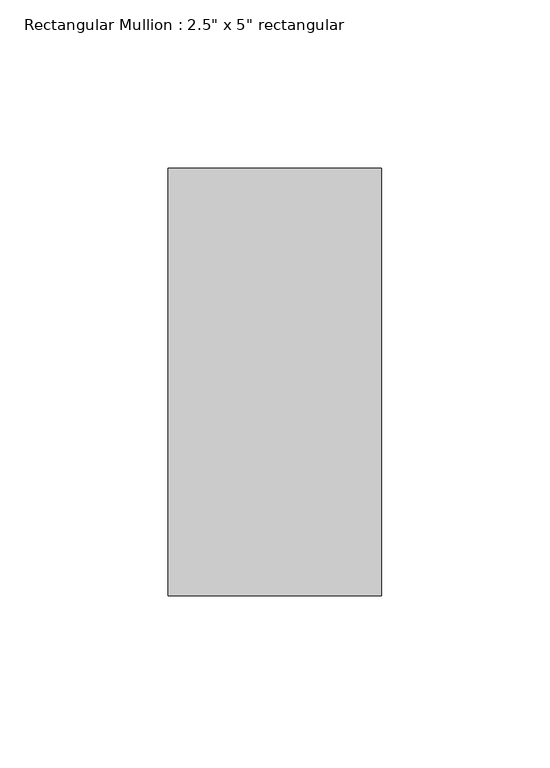
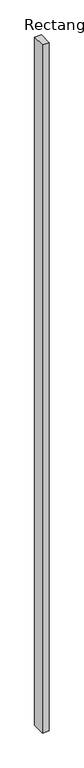
"""IFC4 building model written with IfcOpenShell, lengths in millimetres: member geometry."""

from ifc_helpers import new_model, si_unit, frame, origin, place, context, project, spatial, polyline, outline, extrude, source, transform, mapped, element, save


def member_2b438bbf(model_context):
    return source(origin(), model_context, "Body", "SweptSolid", [
        extrude(outline(polyline([(0.0, 63.5), (0.0, -63.5), (-63.5, -63.5), (-63.5, 63.5), (0.0, 63.5)])), frame((0.0, 0.0, -6966.7943709), z_axis=(0.0, 0.0, 1.0), x_axis=(1.0, 0.0, 0.0)), (0.0, 0.0, 1.0), 6966.7943709),
    ])


if __name__ == "__main__":
    model = new_model("IFC4")
    model_context = context("Model", 3, world=origin())
    ifc_project = project(units=[si_unit("LENGTHUNIT", "METRE", prefix="MILLI")], contexts=[model_context])
    site = spatial("IfcSite", under=ifc_project)
    building = spatial("IfcBuilding", under=site)
    placement = place(None, origin())
    member_shape = member_2b438bbf(model_context)
    element("IfcMember", 1, ObjectType="Rectangular Mullion : 2.5\" x 5\" rectangular", at=placement, inside=building, context=model_context, shape_type="MappedRepresentation", body=[
        mapped(member_shape, transform((0.0, 0.0, 0.0), x_axis=(1.0, 0.0, 0.0), y_axis=(0.0, 1.0, 0.0), z_axis=(0.0, 0.0, 1.0))),
    ])
    save(model, "model.ifc")

# Revit data of these elements
# Type "Rectangular Mullion : 2.5\" x 5\" rectangular"
#   built-in parameter 1007304 = 0.416667 (stored number, unit not read)
#   built-in parameter 1007301 = 0.104167 (stored number, unit not read)
#   built-in parameter 1007300 = 0.104167 (stored number, unit not read)
# Element 1 (IfcMember, "Rectangular Mullion : 2.5\" x 5\" rectangular")
#   Materials on its faces: "Aluminum"
# Materials
#   "Aluminum": class "Metal", colour RGB 247 247 247, transparency 0, Description = "Aluminum 6061", Cost = 0
